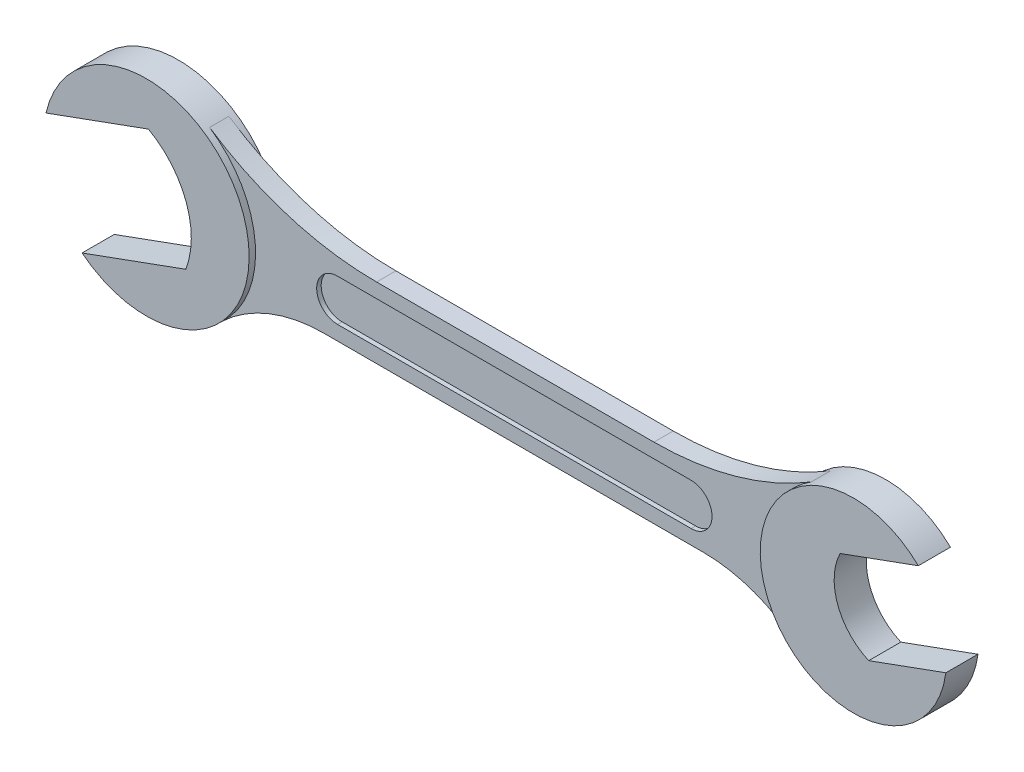
ISO-10303-21;
HEADER;
FILE_DESCRIPTION(('STEP AP214'),'2;1');
FILE_NAME('part.step','',(''),(''),'','','');
FILE_SCHEMA(('AUTOMOTIVE_DESIGN { 1 0 10303 214 1 1 1 1 }'));
ENDSEC;
DATA;
#1=APPLICATION_CONTEXT('core data for automotive mechanical design processes');
#2=APPLICATION_PROTOCOL_DEFINITION('international standard','automotive_design',2000,#1);
#3=PRODUCT_CONTEXT('',#1,'mechanical');
#4=PRODUCT('Part','Part','',(#3));
#5=PRODUCT_RELATED_PRODUCT_CATEGORY('part','',(#4));
#6=PRODUCT_DEFINITION_FORMATION('','',#4);
#7=PRODUCT_DEFINITION_CONTEXT('part definition',#1,'design');
#8=PRODUCT_DEFINITION('design','',#6,#7);
#9=PRODUCT_DEFINITION_SHAPE('','',#8);
#10=(LENGTH_UNIT() NAMED_UNIT(*) SI_UNIT(.MILLI.,.METRE.));
#11=(NAMED_UNIT(*) PLANE_ANGLE_UNIT() SI_UNIT($,.RADIAN.));
#12=(NAMED_UNIT(*) SI_UNIT($,.STERADIAN.) SOLID_ANGLE_UNIT());
#13=UNCERTAINTY_MEASURE_WITH_UNIT(LENGTH_MEASURE(1.E-05),#10,'distance_accuracy_value','');
#14=(GEOMETRIC_REPRESENTATION_CONTEXT(3) GLOBAL_UNCERTAINTY_ASSIGNED_CONTEXT((#13)) GLOBAL_UNIT_ASSIGNED_CONTEXT((#10,
#11,#12)) REPRESENTATION_CONTEXT('',''));
#15=CARTESIAN_POINT('',(0.,0.,0.));
#16=DIRECTION('',(0.,0.,1.));
#17=DIRECTION('',(1.,0.,0.));
#18=AXIS2_PLACEMENT_3D('',#15,#16,#17);
#19=CARTESIAN_POINT('',(0.,0.,3.));
#20=DIRECTION('',(0.,0.,1.));
#21=DIRECTION('',(1.,0.,0.));
#22=AXIS2_PLACEMENT_3D('',#19,#20,#21);
#23=PLANE('',#22);
#24=CARTESIAN_POINT('',(83.7536685908511,0.,3.));
#25=DIRECTION('',(0.,0.,1.));
#26=DIRECTION('',(1.,0.,0.));
#27=AXIS2_PLACEMENT_3D('',#24,#25,#26);
#28=CIRCLE('',#27,3.25);
#29=CARTESIAN_POINT('',(83.7536685908511,-3.25,3.));
#30=VERTEX_POINT('',#29);
#31=CARTESIAN_POINT('',(83.7536685908511,3.25,3.));
#32=VERTEX_POINT('',#31);
#33=EDGE_CURVE('E66',#30,#32,#28,.T.);
#34=ORIENTED_EDGE('',*,*,#33,.F.);
#35=DIRECTION('',(0.99999999999983,5.83857538673517E-07,0.));
#36=VECTOR('',#35,1.);
#37=CARTESIAN_POINT('',(83.7536685908511,-3.25,3.));
#38=LINE('',#37,#36);
#39=CARTESIAN_POINT('',(28.7536685908511,-3.25003211216463,3.));
#40=VERTEX_POINT('',#39);
#41=EDGE_CURVE('E241',#40,#30,#38,.T.);
#42=ORIENTED_EDGE('',*,*,#41,.F.);
#43=CARTESIAN_POINT('',(28.7536685908511,0.,3.));
#44=DIRECTION('',(0.,0.,1.));
#45=DIRECTION('',(1.,0.,0.));
#46=AXIS2_PLACEMENT_3D('',#43,#44,#45);
#47=CIRCLE('',#46,3.25003211216463);
#48=CARTESIAN_POINT('',(28.7681160854874,3.25,3.));
#49=VERTEX_POINT('',#48);
#50=EDGE_CURVE('E259',#49,#40,#47,.T.);
#51=ORIENTED_EDGE('',*,*,#50,.F.);
#52=DIRECTION('',(-1.,0.,0.));
#53=VECTOR('',#52,1.);
#54=CARTESIAN_POINT('',(28.7681160854874,3.25,3.));
#55=LINE('',#54,#53);
#56=EDGE_CURVE('E258',#32,#49,#55,.T.);
#57=ORIENTED_EDGE('',*,*,#56,.F.);
#58=EDGE_LOOP('',(#34,#42,#51,#57));
#59=FACE_BOUND('',#58,.T.);
#60=CARTESIAN_POINT('',(85.6278847860921,-28.5,3.));
#61=DIRECTION('',(0.,0.,1.));
#62=DIRECTION('',(1.,0.,0.));
#63=AXIS2_PLACEMENT_3D('',#60,#61,#62);
#64=CIRCLE('',#63,23.);
#65=CARTESIAN_POINT('',(100.576115450622,-11.02,3.));
#66=VERTEX_POINT('',#65);
#67=CARTESIAN_POINT('',(85.6278847860921,-5.5,3.));
#68=VERTEX_POINT('',#67);
#69=EDGE_CURVE('E341',#66,#68,#64,.T.);
#70=ORIENTED_EDGE('',*,*,#69,.F.);
#71=CARTESIAN_POINT('',(110.,0.,3.));
#72=DIRECTION('',(0.,0.,1.));
#73=DIRECTION('',(1.,0.,0.));
#74=AXIS2_PLACEMENT_3D('',#71,#72,#73);
#75=CIRCLE('',#74,14.5);
#76=CARTESIAN_POINT('',(102.447920260758,12.3780487804878,3.));
#77=VERTEX_POINT('',#76);
#78=EDGE_CURVE('E11',#66,#77,#75,.F.);
#79=ORIENTED_EDGE('',*,*,#78,.T.);
#80=CARTESIAN_POINT('',(77.9687652439061,52.5,3.));
#81=DIRECTION('',(0.,0.,1.));
#82=DIRECTION('',(1.,0.,0.));
#83=AXIS2_PLACEMENT_3D('',#80,#81,#82);
#84=CIRCLE('',#83,47.);
#85=CARTESIAN_POINT('',(77.9687652439086,5.5,3.));
#86=VERTEX_POINT('',#85);
#87=EDGE_CURVE('E327',#77,#86,#84,.F.);
#88=ORIENTED_EDGE('',*,*,#87,.T.);
#89=DIRECTION('',(1.,0.,0.));
#90=VECTOR('',#89,1.);
#91=CARTESIAN_POINT('',(0.,5.5,3.));
#92=LINE('',#91,#90);
#93=CARTESIAN_POINT('',(34.8245602987317,5.5,3.));
#94=VERTEX_POINT('',#93);
#95=EDGE_CURVE('E329',#94,#86,#92,.T.);
#96=ORIENTED_EDGE('',*,*,#95,.F.);
#97=CARTESIAN_POINT('',(34.8245602987317,52.5,3.));
#98=DIRECTION('',(0.,0.,1.));
#99=DIRECTION('',(1.,0.,0.));
#100=AXIS2_PLACEMENT_3D('',#97,#98,#99);
#101=CIRCLE('',#100,47.);
#102=CARTESIAN_POINT('',(8.84433277428107,13.3333333333333,3.));
#103=VERTEX_POINT('',#102);
#104=EDGE_CURVE('E331',#94,#103,#101,.F.);
#105=ORIENTED_EDGE('',*,*,#104,.T.);
#106=CARTESIAN_POINT('',(0.,0.,3.));
#107=DIRECTION('',(0.,0.,1.));
#108=DIRECTION('',(1.,0.,0.));
#109=AXIS2_PLACEMENT_3D('',#106,#107,#108);
#110=CIRCLE('',#109,16.);
#111=CARTESIAN_POINT('',(10.9219934457224,-11.6923076923077,3.));
#112=VERTEX_POINT('',#111);
#113=EDGE_CURVE('E315',#112,#103,#110,.T.);
#114=ORIENTED_EDGE('',*,*,#113,.F.);
#115=CARTESIAN_POINT('',(26.6223590239483,-28.5,3.));
#116=DIRECTION('',(0.,0.,1.));
#117=DIRECTION('',(1.,0.,0.));
#118=AXIS2_PLACEMENT_3D('',#115,#116,#117);
#119=CIRCLE('',#118,23.);
#120=CARTESIAN_POINT('',(26.6223590239447,-5.5,3.));
#121=VERTEX_POINT('',#120);
#122=EDGE_CURVE('E337',#121,#112,#119,.T.);
#123=ORIENTED_EDGE('',*,*,#122,.F.);
#124=DIRECTION('',(1.,0.,0.));
#125=VECTOR('',#124,1.);
#126=CARTESIAN_POINT('',(0.,-5.5,3.));
#127=LINE('',#126,#125);
#128=EDGE_CURVE('E339',#121,#68,#127,.T.);
#129=ORIENTED_EDGE('',*,*,#128,.T.);
#130=EDGE_LOOP('',(#70,#79,#88,#96,#105,#114,#123,#129));
#131=FACE_BOUND('',#130,.T.);
#132=ADVANCED_FACE('F43',(#59,#131),#23,.T.);
#133=CARTESIAN_POINT('',(0.,0.,0.));
#134=DIRECTION('',(0.,0.,1.));
#135=DIRECTION('',(1.,0.,0.));
#136=AXIS2_PLACEMENT_3D('',#133,#134,#135);
#137=PLANE('',#136);
#138=DIRECTION('',(-1.,0.,0.));
#139=VECTOR('',#138,1.);
#140=CARTESIAN_POINT('',(83.6251219050184,-3.24999999999999,0.));
#141=LINE('',#140,#139);
#142=CARTESIAN_POINT('',(83.6251219050184,-3.24999999999999,0.));
#143=VERTEX_POINT('',#142);
#144=CARTESIAN_POINT('',(28.6251219050184,-3.25,0.));
#145=VERTEX_POINT('',#144);
#146=EDGE_CURVE('E235',#143,#145,#141,.T.);
#147=ORIENTED_EDGE('',*,*,#146,.F.);
#148=CARTESIAN_POINT('',(83.6251219050184,0.,0.));
#149=DIRECTION('',(0.,0.,-1.));
#150=DIRECTION('',(-1.,0.,0.));
#151=AXIS2_PLACEMENT_3D('',#148,#149,#150);
#152=CIRCLE('',#151,3.24999999999999);
#153=CARTESIAN_POINT('',(83.6251219050184,3.24999999999999,0.));
#154=VERTEX_POINT('',#153);
#155=EDGE_CURVE('E59',#154,#143,#152,.T.);
#156=ORIENTED_EDGE('',*,*,#155,.F.);
#157=DIRECTION('',(1.,0.,0.));
#158=VECTOR('',#157,1.);
#159=CARTESIAN_POINT('',(83.6251219050184,3.24999999999999,0.));
#160=LINE('',#159,#158);
#161=CARTESIAN_POINT('',(28.6251219050184,3.25,0.));
#162=VERTEX_POINT('',#161);
#163=EDGE_CURVE('E224',#162,#154,#160,.T.);
#164=ORIENTED_EDGE('',*,*,#163,.F.);
#165=CARTESIAN_POINT('',(28.6251219050184,0.,0.));
#166=DIRECTION('',(0.,0.,-1.));
#167=DIRECTION('',(-1.,0.,0.));
#168=AXIS2_PLACEMENT_3D('',#165,#166,#167);
#169=CIRCLE('',#168,3.25);
#170=EDGE_CURVE('E227',#145,#162,#169,.T.);
#171=ORIENTED_EDGE('',*,*,#170,.F.);
#172=EDGE_LOOP('',(#147,#156,#164,#171));
#173=FACE_BOUND('',#172,.T.);
#174=CARTESIAN_POINT('',(110.,0.,0.));
#175=DIRECTION('',(0.,0.,-1.));
#176=DIRECTION('',(-1.,0.,0.));
#177=AXIS2_PLACEMENT_3D('',#174,#175,#176);
#178=CIRCLE('',#177,14.5);
#179=CARTESIAN_POINT('',(100.576115450622,-11.02,0.));
#180=VERTEX_POINT('',#179);
#181=CARTESIAN_POINT('',(102.447920260758,12.3780487804878,0.));
#182=VERTEX_POINT('',#181);
#183=EDGE_CURVE('E283',#180,#182,#178,.T.);
#184=ORIENTED_EDGE('',*,*,#183,.F.);
#185=CARTESIAN_POINT('',(85.6278847860921,-28.5,0.));
#186=DIRECTION('',(0.,0.,1.));
#187=DIRECTION('',(1.,0.,0.));
#188=AXIS2_PLACEMENT_3D('',#185,#186,#187);
#189=CIRCLE('',#188,23.);
#190=CARTESIAN_POINT('',(85.6278847860921,-5.5,0.));
#191=VERTEX_POINT('',#190);
#192=EDGE_CURVE('E332',#180,#191,#189,.T.);
#193=ORIENTED_EDGE('',*,*,#192,.T.);
#194=DIRECTION('',(1.,0.,0.));
#195=VECTOR('',#194,1.);
#196=CARTESIAN_POINT('',(0.,-5.5,0.));
#197=LINE('',#196,#195);
#198=CARTESIAN_POINT('',(26.6223590239447,-5.5,0.));
#199=VERTEX_POINT('',#198);
#200=EDGE_CURVE('E356',#199,#191,#197,.T.);
#201=ORIENTED_EDGE('',*,*,#200,.F.);
#202=CARTESIAN_POINT('',(26.6223590239483,-28.5,0.));
#203=DIRECTION('',(0.,0.,1.));
#204=DIRECTION('',(1.,0.,0.));
#205=AXIS2_PLACEMENT_3D('',#202,#203,#204);
#206=CIRCLE('',#205,23.);
#207=CARTESIAN_POINT('',(10.9219934457224,-11.6923076923077,0.));
#208=VERTEX_POINT('',#207);
#209=EDGE_CURVE('E353',#199,#208,#206,.T.);
#210=ORIENTED_EDGE('',*,*,#209,.T.);
#211=CARTESIAN_POINT('',(0.,0.,0.));
#212=DIRECTION('',(0.,0.,-1.));
#213=DIRECTION('',(-1.,0.,0.));
#214=AXIS2_PLACEMENT_3D('',#211,#212,#213);
#215=CIRCLE('',#214,16.);
#216=CARTESIAN_POINT('',(8.84433277428106,13.3333333333333,0.));
#217=VERTEX_POINT('',#216);
#218=EDGE_CURVE('E51',#217,#208,#215,.T.);
#219=ORIENTED_EDGE('',*,*,#218,.F.);
#220=CARTESIAN_POINT('',(34.8245602987317,52.5,0.));
#221=DIRECTION('',(0.,0.,1.));
#222=DIRECTION('',(1.,0.,0.));
#223=AXIS2_PLACEMENT_3D('',#220,#221,#222);
#224=CIRCLE('',#223,47.);
#225=CARTESIAN_POINT('',(34.8245602987317,5.5,0.));
#226=VERTEX_POINT('',#225);
#227=EDGE_CURVE('E348',#226,#217,#224,.F.);
#228=ORIENTED_EDGE('',*,*,#227,.F.);
#229=DIRECTION('',(1.,0.,0.));
#230=VECTOR('',#229,1.);
#231=CARTESIAN_POINT('',(0.,5.5,0.));
#232=LINE('',#231,#230);
#233=CARTESIAN_POINT('',(77.9687652439086,5.5,0.));
#234=VERTEX_POINT('',#233);
#235=EDGE_CURVE('E350',#226,#234,#232,.T.);
#236=ORIENTED_EDGE('',*,*,#235,.T.);
#237=CARTESIAN_POINT('',(77.9687652439061,52.5,0.));
#238=DIRECTION('',(0.,0.,1.));
#239=DIRECTION('',(1.,0.,0.));
#240=AXIS2_PLACEMENT_3D('',#237,#238,#239);
#241=CIRCLE('',#240,47.);
#242=EDGE_CURVE('E322',#182,#234,#241,.F.);
#243=ORIENTED_EDGE('',*,*,#242,.F.);
#244=EDGE_LOOP('',(#184,#193,#201,#210,#219,#228,#236,#243));
#245=FACE_BOUND('',#244,.T.);
#246=ADVANCED_FACE('F422',(#173,#245),#137,.F.);
#247=CARTESIAN_POINT('',(10.7035037567005,-29.4076348820317,3.));
#248=DIRECTION('',(0.342020143310785,-0.939692620791326,0.));
#249=DIRECTION('',(0.939692620791326,0.342020143310785,0.));
#250=AXIS2_PLACEMENT_3D('',#247,#248,#249);
#251=PLANE('',#250);
#252=DIRECTION('',(0.,0.,-1.));
#253=VECTOR('',#252,1.);
#254=CARTESIAN_POINT('',(107.927329676916,5.97894381266167,3.));
#255=LINE('',#254,#253);
#256=CARTESIAN_POINT('',(107.927329676916,5.97894381266167,4.));
#257=VERTEX_POINT('',#256);
#258=CARTESIAN_POINT('',(107.927329676916,5.97894381266167,-1.));
#259=VERTEX_POINT('',#258);
#260=EDGE_CURVE('E343',#257,#259,#255,.T.);
#261=ORIENTED_EDGE('',*,*,#260,.T.);
#262=DIRECTION('',(-0.939692620791326,-0.342020143310785,0.));
#263=VECTOR('',#262,1.);
#264=CARTESIAN_POINT('',(107.927329676916,5.97894381266167,-1.));
#265=LINE('',#264,#263);
#266=CARTESIAN_POINT('',(120.095812240616,10.4079092618175,-1.));
#267=VERTEX_POINT('',#266);
#268=EDGE_CURVE('E291',#267,#259,#265,.T.);
#269=ORIENTED_EDGE('',*,*,#268,.F.);
#270=DIRECTION('',(0.,0.,-1.));
#271=VECTOR('',#270,1.);
#272=CARTESIAN_POINT('',(120.095812240616,10.4079092618175,3.));
#273=LINE('',#272,#271);
#274=CARTESIAN_POINT('',(120.095812240616,10.4079092618175,4.));
#275=VERTEX_POINT('',#274);
#276=EDGE_CURVE('E330',#275,#267,#273,.T.);
#277=ORIENTED_EDGE('',*,*,#276,.F.);
#278=DIRECTION('',(0.939692620791326,0.342020143310785,0.));
#279=VECTOR('',#278,1.);
#280=CARTESIAN_POINT('',(107.927329676916,5.97894381266167,4.));
#281=LINE('',#280,#279);
#282=EDGE_CURVE('E273',#257,#275,#281,.T.);
#283=ORIENTED_EDGE('',*,*,#282,.F.);
#284=EDGE_LOOP('',(#261,#269,#277,#283));
#285=FACE_BOUND('',#284,.T.);
#286=ADVANCED_FACE('F44',(#285),#251,.T.);
#287=CARTESIAN_POINT('',(77.9687652439061,52.5,3.));
#288=DIRECTION('',(0.,0.,-1.));
#289=DIRECTION('',(-1.,0.,0.));
#290=AXIS2_PLACEMENT_3D('',#287,#288,#289);
#291=CYLINDRICAL_SURFACE('',#290,47.);
#292=ORIENTED_EDGE('',*,*,#242,.T.);
#293=DIRECTION('',(0.,0.,-1.));
#294=VECTOR('',#293,1.);
#295=CARTESIAN_POINT('',(77.9687652439086,5.5,3.));
#296=LINE('',#295,#294);
#297=EDGE_CURVE('E386',#86,#234,#296,.T.);
#298=ORIENTED_EDGE('',*,*,#297,.F.);
#299=ORIENTED_EDGE('',*,*,#87,.F.);
#300=DIRECTION('',(0.,0.,-1.));
#301=VECTOR('',#300,1.);
#302=CARTESIAN_POINT('',(102.447920260758,12.3780487804878,3.));
#303=LINE('',#302,#301);
#304=EDGE_CURVE('E392',#77,#182,#303,.T.);
#305=ORIENTED_EDGE('',*,*,#304,.T.);
#306=EDGE_LOOP('',(#292,#298,#299,#305));
#307=FACE_BOUND('',#306,.T.);
#308=ADVANCED_FACE('F480',(#307),#291,.F.);
#309=CARTESIAN_POINT('',(0.,5.5,3.));
#310=DIRECTION('',(0.,1.,0.));
#311=DIRECTION('',(0.,0.,1.));
#312=AXIS2_PLACEMENT_3D('',#309,#310,#311);
#313=PLANE('',#312);
#314=ORIENTED_EDGE('',*,*,#235,.F.);
#315=DIRECTION('',(0.,0.,-1.));
#316=VECTOR('',#315,1.);
#317=CARTESIAN_POINT('',(34.8245602987317,5.5,3.));
#318=LINE('',#317,#316);
#319=EDGE_CURVE('E390',#94,#226,#318,.T.);
#320=ORIENTED_EDGE('',*,*,#319,.F.);
#321=ORIENTED_EDGE('',*,*,#95,.T.);
#322=ORIENTED_EDGE('',*,*,#297,.T.);
#323=EDGE_LOOP('',(#314,#320,#321,#322));
#324=FACE_BOUND('',#323,.T.);
#325=ADVANCED_FACE('F475',(#324),#313,.T.);
#326=CARTESIAN_POINT('',(34.8245602987317,52.5,3.));
#327=DIRECTION('',(0.,0.,-1.));
#328=DIRECTION('',(-1.,0.,0.));
#329=AXIS2_PLACEMENT_3D('',#326,#327,#328);
#330=CYLINDRICAL_SURFACE('',#329,47.);
#331=ORIENTED_EDGE('',*,*,#227,.T.);
#332=DIRECTION('',(0.,0.,-1.));
#333=VECTOR('',#332,1.);
#334=CARTESIAN_POINT('',(8.84433277428107,13.3333333333333,3.));
#335=LINE('',#334,#333);
#336=EDGE_CURVE('E383',#103,#217,#335,.T.);
#337=ORIENTED_EDGE('',*,*,#336,.F.);
#338=ORIENTED_EDGE('',*,*,#104,.F.);
#339=ORIENTED_EDGE('',*,*,#319,.T.);
#340=EDGE_LOOP('',(#331,#337,#338,#339));
#341=FACE_BOUND('',#340,.T.);
#342=ADVANCED_FACE('F469',(#341),#330,.F.);
#343=CARTESIAN_POINT('',(-2.96625027922472,8.14970566262087,3.));
#344=DIRECTION('',(-0.34202014332567,0.939692620785908,0.));
#345=DIRECTION('',(-0.939692620785908,-0.34202014332567,0.));
#346=AXIS2_PLACEMENT_3D('',#343,#344,#345);
#347=PLANE('',#346);
#348=DIRECTION('',(0.,0.,-1.));
#349=VECTOR('',#348,1.);
#350=CARTESIAN_POINT('',(-15.6009638229452,3.55104601422654,3.));
#351=LINE('',#350,#349);
#352=CARTESIAN_POINT('',(-15.6009638229452,3.55104601422654,4.));
#353=VERTEX_POINT('',#352);
#354=CARTESIAN_POINT('',(-15.6009638229452,3.55104601422654,-1.));
#355=VERTEX_POINT('',#354);
#356=EDGE_CURVE('E385',#353,#355,#351,.T.);
#357=ORIENTED_EDGE('',*,*,#356,.T.);
#358=DIRECTION('',(-0.939692620785908,-0.34202014332567,0.));
#359=VECTOR('',#358,1.);
#360=CARTESIAN_POINT('',(0.335793670547545,9.35155137257678,-1.));
#361=LINE('',#360,#359);
#362=CARTESIAN_POINT('',(0.335793670547545,9.35155137257678,-1.));
#363=VERTEX_POINT('',#362);
#364=EDGE_CURVE('E301',#363,#355,#361,.T.);
#365=ORIENTED_EDGE('',*,*,#364,.F.);
#366=DIRECTION('',(0.,0.,-1.));
#367=VECTOR('',#366,1.);
#368=CARTESIAN_POINT('',(0.335793670547545,9.35155137257678,3.));
#369=LINE('',#368,#367);
#370=CARTESIAN_POINT('',(0.335793670547545,9.35155137257678,4.));
#371=VERTEX_POINT('',#370);
#372=EDGE_CURVE('E379',#371,#363,#369,.T.);
#373=ORIENTED_EDGE('',*,*,#372,.F.);
#374=DIRECTION('',(0.939692620785908,0.34202014332567,0.));
#375=VECTOR('',#374,1.);
#376=CARTESIAN_POINT('',(-15.6009638229452,3.55104601422654,4.));
#377=LINE('',#376,#375);
#378=EDGE_CURVE('E312',#353,#371,#377,.T.);
#379=ORIENTED_EDGE('',*,*,#378,.F.);
#380=EDGE_LOOP('',(#357,#365,#373,#379));
#381=FACE_BOUND('',#380,.T.);
#382=ADVANCED_FACE('F466',(#381),#347,.F.);
#383=CARTESIAN_POINT('',(-6.,-2.,3.));
#384=DIRECTION('',(0.,0.,-1.));
#385=DIRECTION('',(-1.,0.,0.));
#386=AXIS2_PLACEMENT_3D('',#383,#384,#385);
#387=CYLINDRICAL_SURFACE('',#386,13.);
#388=ORIENTED_EDGE('',*,*,#372,.T.);
#389=CARTESIAN_POINT('',(-6.,-2.,-1.));
#390=DIRECTION('',(0.,0.,1.));
#391=DIRECTION('',(1.,0.,0.));
#392=AXIS2_PLACEMENT_3D('',#389,#390,#391);
#393=CIRCLE('',#392,13.);
#394=CARTESIAN_POINT('',(6.15013610708393,-6.62322318078366,-1.));
#395=VERTEX_POINT('',#394);
#396=EDGE_CURVE('E297',#395,#363,#393,.T.);
#397=ORIENTED_EDGE('',*,*,#396,.F.);
#398=DIRECTION('',(0.,0.,-1.));
#399=VECTOR('',#398,1.);
#400=CARTESIAN_POINT('',(6.15013610708393,-6.62322318078366,3.));
#401=LINE('',#400,#399);
#402=CARTESIAN_POINT('',(6.15013610708393,-6.62322318078366,4.));
#403=VERTEX_POINT('',#402);
#404=EDGE_CURVE('E378',#403,#395,#401,.T.);
#405=ORIENTED_EDGE('',*,*,#404,.F.);
#406=CARTESIAN_POINT('',(-6.00000000000002,-2.,4.));
#407=DIRECTION('',(0.,0.,-1.));
#408=DIRECTION('',(-1.,0.,0.));
#409=AXIS2_PLACEMENT_3D('',#406,#407,#408);
#410=CIRCLE('',#409,13.);
#411=EDGE_CURVE('E318',#371,#403,#410,.T.);
#412=ORIENTED_EDGE('',*,*,#411,.F.);
#413=EDGE_LOOP('',(#388,#397,#405,#412));
#414=FACE_BOUND('',#413,.T.);
#415=ADVANCED_FACE('F465',(#414),#387,.F.);
#416=CARTESIAN_POINT('',(2.84809215731166,-7.82506889073957,3.));
#417=DIRECTION('',(0.342020143325669,-0.939692620785908,0.));
#418=DIRECTION('',(0.939692620785908,0.342020143325669,0.));
#419=AXIS2_PLACEMENT_3D('',#416,#417,#418);
#420=PLANE('',#419);
#421=ORIENTED_EDGE('',*,*,#404,.T.);
#422=DIRECTION('',(0.939692620785908,0.342020143325669,0.));
#423=VECTOR('',#422,1.);
#424=CARTESIAN_POINT('',(6.15013610708393,-6.62322318078366,-1.));
#425=LINE('',#424,#423);
#426=CARTESIAN_POINT('',(-9.99020934928993,-12.4978284976775,-1.));
#427=VERTEX_POINT('',#426);
#428=EDGE_CURVE('E307',#427,#395,#425,.T.);
#429=ORIENTED_EDGE('',*,*,#428,.F.);
#430=DIRECTION('',(0.,0.,-1.));
#431=VECTOR('',#430,1.);
#432=CARTESIAN_POINT('',(-9.99020934928993,-12.4978284976775,3.));
#433=LINE('',#432,#431);
#434=CARTESIAN_POINT('',(-9.99020934928993,-12.4978284976775,4.));
#435=VERTEX_POINT('',#434);
#436=EDGE_CURVE('E376',#435,#427,#433,.T.);
#437=ORIENTED_EDGE('',*,*,#436,.F.);
#438=DIRECTION('',(-0.939692620785908,-0.342020143325669,0.));
#439=VECTOR('',#438,1.);
#440=CARTESIAN_POINT('',(-9.99020934928993,-12.4978284976775,4.));
#441=LINE('',#440,#439);
#442=EDGE_CURVE('E321',#403,#435,#441,.T.);
#443=ORIENTED_EDGE('',*,*,#442,.F.);
#444=EDGE_LOOP('',(#421,#429,#437,#443));
#445=FACE_BOUND('',#444,.T.);
#446=ADVANCED_FACE('F456',(#445),#420,.F.);
#447=CARTESIAN_POINT('',(0.,0.,3.));
#448=DIRECTION('',(0.,0.,-1.));
#449=DIRECTION('',(-1.,0.,0.));
#450=AXIS2_PLACEMENT_3D('',#447,#448,#449);
#451=CYLINDRICAL_SURFACE('',#450,16.);
#452=CARTESIAN_POINT('',(0.,0.,-1.));
#453=DIRECTION('',(0.,0.,-1.));
#454=DIRECTION('',(-1.,0.,0.));
#455=AXIS2_PLACEMENT_3D('',#452,#453,#454);
#456=CIRCLE('',#455,16.);
#457=EDGE_CURVE('E303',#355,#427,#456,.T.);
#458=ORIENTED_EDGE('',*,*,#457,.F.);
#459=ORIENTED_EDGE('',*,*,#356,.F.);
#460=CARTESIAN_POINT('',(0.,0.,4.));
#461=DIRECTION('',(0.,0.,1.));
#462=DIRECTION('',(1.,0.,0.));
#463=AXIS2_PLACEMENT_3D('',#460,#461,#462);
#464=CIRCLE('',#463,16.);
#465=EDGE_CURVE('E309',#435,#353,#464,.T.);
#466=ORIENTED_EDGE('',*,*,#465,.F.);
#467=ORIENTED_EDGE('',*,*,#436,.T.);
#468=EDGE_LOOP('',(#458,#459,#466,#467));
#469=FACE_BOUND('',#468,.T.);
#470=ORIENTED_EDGE('',*,*,#336,.T.);
#471=ORIENTED_EDGE('',*,*,#218,.T.);
#472=DIRECTION('',(0.,0.,-1.));
#473=VECTOR('',#472,1.);
#474=CARTESIAN_POINT('',(10.9219934457224,-11.6923076923077,3.));
#475=LINE('',#474,#473);
#476=EDGE_CURVE('E373',#112,#208,#475,.T.);
#477=ORIENTED_EDGE('',*,*,#476,.F.);
#478=ORIENTED_EDGE('',*,*,#113,.T.);
#479=EDGE_LOOP('',(#470,#471,#477,#478));
#480=FACE_BOUND('',#479,.T.);
#481=ADVANCED_FACE('F453',(#469,#480),#451,.T.);
#482=CARTESIAN_POINT('',(26.6223590239483,-28.5,3.));
#483=DIRECTION('',(0.,0.,-1.));
#484=DIRECTION('',(-1.,0.,0.));
#485=AXIS2_PLACEMENT_3D('',#482,#483,#484);
#486=CYLINDRICAL_SURFACE('',#485,23.);
#487=ORIENTED_EDGE('',*,*,#209,.F.);
#488=DIRECTION('',(0.,0.,-1.));
#489=VECTOR('',#488,1.);
#490=CARTESIAN_POINT('',(26.6223590239447,-5.5,3.));
#491=LINE('',#490,#489);
#492=EDGE_CURVE('E371',#121,#199,#491,.T.);
#493=ORIENTED_EDGE('',*,*,#492,.F.);
#494=ORIENTED_EDGE('',*,*,#122,.T.);
#495=ORIENTED_EDGE('',*,*,#476,.T.);
#496=EDGE_LOOP('',(#487,#493,#494,#495));
#497=FACE_BOUND('',#496,.T.);
#498=ADVANCED_FACE('F446',(#497),#486,.F.);
#499=CARTESIAN_POINT('',(0.,-5.5,3.));
#500=DIRECTION('',(0.,1.,0.));
#501=DIRECTION('',(-1.,0.,0.));
#502=AXIS2_PLACEMENT_3D('',#499,#500,#501);
#503=PLANE('',#502);
#504=ORIENTED_EDGE('',*,*,#200,.T.);
#505=DIRECTION('',(0.,0.,-1.));
#506=VECTOR('',#505,1.);
#507=CARTESIAN_POINT('',(85.6278847860921,-5.5,3.));
#508=LINE('',#507,#506);
#509=EDGE_CURVE('E369',#68,#191,#508,.T.);
#510=ORIENTED_EDGE('',*,*,#509,.F.);
#511=ORIENTED_EDGE('',*,*,#128,.F.);
#512=ORIENTED_EDGE('',*,*,#492,.T.);
#513=EDGE_LOOP('',(#504,#510,#511,#512));
#514=FACE_BOUND('',#513,.T.);
#515=ADVANCED_FACE('F447',(#514),#503,.F.);
#516=CARTESIAN_POINT('',(85.6278847860921,-28.5,3.));
#517=DIRECTION('',(0.,0.,-1.));
#518=DIRECTION('',(-1.,0.,0.));
#519=AXIS2_PLACEMENT_3D('',#516,#517,#518);
#520=CYLINDRICAL_SURFACE('',#519,23.);
#521=ORIENTED_EDGE('',*,*,#192,.F.);
#522=DIRECTION('',(0.,0.,-1.));
#523=VECTOR('',#522,1.);
#524=CARTESIAN_POINT('',(100.576115450622,-11.02,3.));
#525=LINE('',#524,#523);
#526=EDGE_CURVE('E368',#66,#180,#525,.T.);
#527=ORIENTED_EDGE('',*,*,#526,.F.);
#528=ORIENTED_EDGE('',*,*,#69,.T.);
#529=ORIENTED_EDGE('',*,*,#509,.T.);
#530=EDGE_LOOP('',(#521,#527,#528,#529));
#531=FACE_BOUND('',#530,.T.);
#532=ADVANCED_FACE('F444',(#531),#520,.F.);
#533=CARTESIAN_POINT('',(110.,0.,3.));
#534=DIRECTION('',(0.,0.,-1.));
#535=DIRECTION('',(-1.,0.,0.));
#536=AXIS2_PLACEMENT_3D('',#533,#534,#535);
#537=CYLINDRICAL_SURFACE('',#536,14.5);
#538=DIRECTION('',(0.,0.,-1.));
#539=VECTOR('',#538,1.);
#540=CARTESIAN_POINT('',(124.379255247521,-1.86735602567682,3.));
#541=LINE('',#540,#539);
#542=CARTESIAN_POINT('',(124.379255247521,-1.86735602567682,4.));
#543=VERTEX_POINT('',#542);
#544=CARTESIAN_POINT('',(124.379255247521,-1.86735602567682,-1.));
#545=VERTEX_POINT('',#544);
#546=EDGE_CURVE('E365',#543,#545,#541,.T.);
#547=ORIENTED_EDGE('',*,*,#546,.F.);
#548=CARTESIAN_POINT('',(110.,0.,4.));
#549=DIRECTION('',(0.,0.,1.));
#550=DIRECTION('',(1.,0.,0.));
#551=AXIS2_PLACEMENT_3D('',#548,#549,#550);
#552=CIRCLE('',#551,14.5);
#553=EDGE_CURVE('E280',#275,#543,#552,.T.);
#554=ORIENTED_EDGE('',*,*,#553,.F.);
#555=ORIENTED_EDGE('',*,*,#276,.T.);
#556=CARTESIAN_POINT('',(110.,0.,-1.));
#557=DIRECTION('',(0.,0.,-1.));
#558=DIRECTION('',(-1.,0.,0.));
#559=AXIS2_PLACEMENT_3D('',#556,#557,#558);
#560=CIRCLE('',#559,14.5);
#561=EDGE_CURVE('E289',#545,#267,#560,.T.);
#562=ORIENTED_EDGE('',*,*,#561,.F.);
#563=EDGE_LOOP('',(#547,#554,#555,#562));
#564=FACE_BOUND('',#563,.T.);
#565=ORIENTED_EDGE('',*,*,#526,.T.);
#566=ORIENTED_EDGE('',*,*,#183,.T.);
#567=ORIENTED_EDGE('',*,*,#304,.F.);
#568=ORIENTED_EDGE('',*,*,#78,.F.);
#569=EDGE_LOOP('',(#565,#566,#567,#568));
#570=FACE_BOUND('',#569,.T.);
#571=ADVANCED_FACE('F391',(#564,#570),#537,.T.);
#572=CARTESIAN_POINT('',(15.1497656197431,-41.6236389523214,3.));
#573=DIRECTION('',(-0.342020143310813,0.939692620791315,0.));
#574=DIRECTION('',(-0.939692620791316,-0.342020143310813,0.));
#575=AXIS2_PLACEMENT_3D('',#572,#573,#574);
#576=PLANE('',#575);
#577=ORIENTED_EDGE('',*,*,#546,.T.);
#578=DIRECTION('',(0.939692620791316,0.342020143310813,0.));
#579=VECTOR('',#578,1.);
#580=CARTESIAN_POINT('',(112.373591540149,-6.23706025755531,-1.));
#581=LINE('',#580,#579);
#582=CARTESIAN_POINT('',(112.373591540149,-6.23706025755531,-1.));
#583=VERTEX_POINT('',#582);
#584=EDGE_CURVE('E290',#583,#545,#581,.T.);
#585=ORIENTED_EDGE('',*,*,#584,.F.);
#586=DIRECTION('',(0.,0.,-1.));
#587=VECTOR('',#586,1.);
#588=CARTESIAN_POINT('',(112.373591540149,-6.23706025755531,3.));
#589=LINE('',#588,#587);
#590=CARTESIAN_POINT('',(112.373591540149,-6.23706025755531,4.));
#591=VERTEX_POINT('',#590);
#592=EDGE_CURVE('E362',#591,#583,#589,.T.);
#593=ORIENTED_EDGE('',*,*,#592,.F.);
#594=DIRECTION('',(-0.939692620791316,-0.342020143310813,0.));
#595=VECTOR('',#594,1.);
#596=CARTESIAN_POINT('',(112.373591540149,-6.23706025755531,4.));
#597=LINE('',#596,#595);
#598=EDGE_CURVE('E278',#543,#591,#597,.T.);
#599=ORIENTED_EDGE('',*,*,#598,.F.);
#600=EDGE_LOOP('',(#577,#585,#593,#599));
#601=FACE_BOUND('',#600,.T.);
#602=ADVANCED_FACE('F409',(#601),#576,.T.);
#603=CARTESIAN_POINT('',(115.99999999941,2.0000000000001,3.));
#604=DIRECTION('',(0.,0.,-1.));
#605=DIRECTION('',(-1.,0.,0.));
#606=AXIS2_PLACEMENT_3D('',#603,#604,#605);
#607=CYLINDRICAL_SURFACE('',#606,9.);
#608=ORIENTED_EDGE('',*,*,#592,.T.);
#609=CARTESIAN_POINT('',(115.99999999941,2.00000000000009,-1.));
#610=DIRECTION('',(0.,0.,1.));
#611=DIRECTION('',(1.,0.,0.));
#612=AXIS2_PLACEMENT_3D('',#609,#610,#611);
#613=CIRCLE('',#612,9.00000000000001);
#614=EDGE_CURVE('E284',#259,#583,#613,.T.);
#615=ORIENTED_EDGE('',*,*,#614,.F.);
#616=ORIENTED_EDGE('',*,*,#260,.F.);
#617=CARTESIAN_POINT('',(115.99999999941,2.00000000000009,4.));
#618=DIRECTION('',(0.,0.,-1.));
#619=DIRECTION('',(1.,0.,0.));
#620=AXIS2_PLACEMENT_3D('',#617,#618,#619);
#621=CIRCLE('',#620,9.00000000000001);
#622=EDGE_CURVE('E266',#591,#257,#621,.T.);
#623=ORIENTED_EDGE('',*,*,#622,.F.);
#624=EDGE_LOOP('',(#608,#615,#616,#623));
#625=FACE_BOUND('',#624,.T.);
#626=ADVANCED_FACE('F407',(#625),#607,.F.);
#627=CARTESIAN_POINT('',(0.,0.,4.));
#628=DIRECTION('',(0.,0.,1.));
#629=DIRECTION('',(1.,0.,0.));
#630=AXIS2_PLACEMENT_3D('',#627,#628,#629);
#631=PLANE('',#630);
#632=ORIENTED_EDGE('',*,*,#465,.T.);
#633=ORIENTED_EDGE('',*,*,#378,.T.);
#634=ORIENTED_EDGE('',*,*,#411,.T.);
#635=ORIENTED_EDGE('',*,*,#442,.T.);
#636=EDGE_LOOP('',(#632,#633,#634,#635));
#637=FACE_BOUND('',#636,.T.);
#638=ADVANCED_FACE('F434',(#637),#631,.T.);
#639=CARTESIAN_POINT('',(-6.,-2.,-1.));
#640=DIRECTION('',(0.,0.,1.));
#641=DIRECTION('',(1.,0.,0.));
#642=AXIS2_PLACEMENT_3D('',#639,#640,#641);
#643=PLANE('',#642);
#644=ORIENTED_EDGE('',*,*,#396,.T.);
#645=ORIENTED_EDGE('',*,*,#364,.T.);
#646=ORIENTED_EDGE('',*,*,#457,.T.);
#647=ORIENTED_EDGE('',*,*,#428,.T.);
#648=EDGE_LOOP('',(#644,#645,#646,#647));
#649=FACE_BOUND('',#648,.T.);
#650=ADVANCED_FACE('F421',(#649),#643,.F.);
#651=CARTESIAN_POINT('',(115.99999999941,2.00000000000009,-1.));
#652=DIRECTION('',(0.,0.,1.));
#653=DIRECTION('',(1.,0.,0.));
#654=AXIS2_PLACEMENT_3D('',#651,#652,#653);
#655=PLANE('',#654);
#656=ORIENTED_EDGE('',*,*,#614,.T.);
#657=ORIENTED_EDGE('',*,*,#584,.T.);
#658=ORIENTED_EDGE('',*,*,#561,.T.);
#659=ORIENTED_EDGE('',*,*,#268,.T.);
#660=EDGE_LOOP('',(#656,#657,#658,#659));
#661=FACE_BOUND('',#660,.T.);
#662=ADVANCED_FACE('F402',(#661),#655,.F.);
#663=CARTESIAN_POINT('',(115.99999999941,2.00000000000009,4.));
#664=DIRECTION('',(0.,0.,1.));
#665=DIRECTION('',(1.,0.,0.));
#666=AXIS2_PLACEMENT_3D('',#663,#664,#665);
#667=PLANE('',#666);
#668=ORIENTED_EDGE('',*,*,#622,.T.);
#669=ORIENTED_EDGE('',*,*,#282,.T.);
#670=ORIENTED_EDGE('',*,*,#553,.T.);
#671=ORIENTED_EDGE('',*,*,#598,.T.);
#672=EDGE_LOOP('',(#668,#669,#670,#671));
#673=FACE_BOUND('',#672,.T.);
#674=ADVANCED_FACE('F411',(#673),#667,.T.);
#675=CARTESIAN_POINT('',(83.7536685908511,0.,2.3));
#676=DIRECTION('',(0.,0.,1.));
#677=DIRECTION('',(1.,0.,0.));
#678=AXIS2_PLACEMENT_3D('',#675,#676,#677);
#679=CYLINDRICAL_SURFACE('',#678,3.25);
#680=ORIENTED_EDGE('',*,*,#33,.T.);
#681=DIRECTION('',(0.,0.,1.));
#682=VECTOR('',#681,1.);
#683=CARTESIAN_POINT('',(83.7536685908511,3.25,2.3));
#684=LINE('',#683,#682);
#685=CARTESIAN_POINT('',(83.7536685908511,3.25,2.3));
#686=VERTEX_POINT('',#685);
#687=EDGE_CURVE('E255',#686,#32,#684,.T.);
#688=ORIENTED_EDGE('',*,*,#687,.F.);
#689=CARTESIAN_POINT('',(83.7536685908511,0.,2.3));
#690=DIRECTION('',(0.,0.,1.));
#691=DIRECTION('',(1.,0.,0.));
#692=AXIS2_PLACEMENT_3D('',#689,#690,#691);
#693=CIRCLE('',#692,3.25);
#694=CARTESIAN_POINT('',(83.7536685908511,-3.25,2.3));
#695=VERTEX_POINT('',#694);
#696=EDGE_CURVE('E242',#695,#686,#693,.T.);
#697=ORIENTED_EDGE('',*,*,#696,.F.);
#698=DIRECTION('',(0.,0.,1.));
#699=VECTOR('',#698,1.);
#700=CARTESIAN_POINT('',(83.7536685908511,-3.25,2.3));
#701=LINE('',#700,#699);
#702=EDGE_CURVE('E262',#695,#30,#701,.T.);
#703=ORIENTED_EDGE('',*,*,#702,.T.);
#704=EDGE_LOOP('',(#680,#688,#697,#703));
#705=FACE_BOUND('',#704,.T.);
#706=ADVANCED_FACE('F412',(#705),#679,.F.);
#707=CARTESIAN_POINT('',(83.7536685908511,-3.25,2.3));
#708=DIRECTION('',(5.83857538673517E-07,-0.999999999999829,0.));
#709=DIRECTION('',(0.99999999999983,5.83857538673517E-07,0.));
#710=AXIS2_PLACEMENT_3D('',#707,#708,#709);
#711=PLANE('',#710);
#712=ORIENTED_EDGE('',*,*,#41,.T.);
#713=ORIENTED_EDGE('',*,*,#702,.F.);
#714=DIRECTION('',(0.99999999999983,5.83857538673517E-07,0.));
#715=VECTOR('',#714,1.);
#716=CARTESIAN_POINT('',(83.7536685908511,-3.25,2.3));
#717=LINE('',#716,#715);
#718=CARTESIAN_POINT('',(28.7536685908511,-3.25003211216463,2.3));
#719=VERTEX_POINT('',#718);
#720=EDGE_CURVE('E253',#719,#695,#717,.T.);
#721=ORIENTED_EDGE('',*,*,#720,.F.);
#722=DIRECTION('',(0.,0.,1.));
#723=VECTOR('',#722,1.);
#724=CARTESIAN_POINT('',(28.7536685908511,-3.25003211216463,2.3));
#725=LINE('',#724,#723);
#726=EDGE_CURVE('E270',#719,#40,#725,.T.);
#727=ORIENTED_EDGE('',*,*,#726,.T.);
#728=EDGE_LOOP('',(#712,#713,#721,#727));
#729=FACE_BOUND('',#728,.T.);
#730=ADVANCED_FACE('F419',(#729),#711,.F.);
#731=CARTESIAN_POINT('',(28.7536685908511,0.,2.3));
#732=DIRECTION('',(0.,0.,1.));
#733=DIRECTION('',(1.,0.,0.));
#734=AXIS2_PLACEMENT_3D('',#731,#732,#733);
#735=CYLINDRICAL_SURFACE('',#734,3.25003211216463);
#736=ORIENTED_EDGE('',*,*,#50,.T.);
#737=ORIENTED_EDGE('',*,*,#726,.F.);
#738=CARTESIAN_POINT('',(28.7536685908511,0.,2.3));
#739=DIRECTION('',(0.,0.,1.));
#740=DIRECTION('',(1.,0.,0.));
#741=AXIS2_PLACEMENT_3D('',#738,#739,#740);
#742=CIRCLE('',#741,3.25003211216463);
#743=CARTESIAN_POINT('',(28.7681160854874,3.25,2.3));
#744=VERTEX_POINT('',#743);
#745=EDGE_CURVE('E247',#744,#719,#742,.T.);
#746=ORIENTED_EDGE('',*,*,#745,.F.);
#747=DIRECTION('',(0.,0.,1.));
#748=VECTOR('',#747,1.);
#749=CARTESIAN_POINT('',(28.7681160854874,3.25,2.3));
#750=LINE('',#749,#748);
#751=EDGE_CURVE('E267',#744,#49,#750,.T.);
#752=ORIENTED_EDGE('',*,*,#751,.T.);
#753=EDGE_LOOP('',(#736,#737,#746,#752));
#754=FACE_BOUND('',#753,.T.);
#755=ADVANCED_FACE('F634',(#754),#735,.F.);
#756=CARTESIAN_POINT('',(28.7681160854874,3.25,2.3));
#757=DIRECTION('',(0.,1.,0.));
#758=DIRECTION('',(0.,0.,1.));
#759=AXIS2_PLACEMENT_3D('',#756,#757,#758);
#760=PLANE('',#759);
#761=ORIENTED_EDGE('',*,*,#56,.T.);
#762=ORIENTED_EDGE('',*,*,#751,.F.);
#763=DIRECTION('',(-1.,0.,0.));
#764=VECTOR('',#763,1.);
#765=CARTESIAN_POINT('',(28.7681160854874,3.25,2.3));
#766=LINE('',#765,#764);
#767=EDGE_CURVE('E244',#686,#744,#766,.T.);
#768=ORIENTED_EDGE('',*,*,#767,.F.);
#769=ORIENTED_EDGE('',*,*,#687,.T.);
#770=EDGE_LOOP('',(#761,#762,#768,#769));
#771=FACE_BOUND('',#770,.T.);
#772=ADVANCED_FACE('F642',(#771),#760,.F.);
#773=CARTESIAN_POINT('',(83.7536685908511,0.,2.3));
#774=DIRECTION('',(0.,0.,1.));
#775=DIRECTION('',(1.,0.,0.));
#776=AXIS2_PLACEMENT_3D('',#773,#774,#775);
#777=PLANE('',#776);
#778=ORIENTED_EDGE('',*,*,#696,.T.);
#779=ORIENTED_EDGE('',*,*,#767,.T.);
#780=ORIENTED_EDGE('',*,*,#745,.T.);
#781=ORIENTED_EDGE('',*,*,#720,.T.);
#782=EDGE_LOOP('',(#778,#779,#780,#781));
#783=FACE_BOUND('',#782,.T.);
#784=ADVANCED_FACE('F654',(#783),#777,.T.);
#785=CARTESIAN_POINT('',(83.6251219050184,0.,0.7));
#786=DIRECTION('',(0.,0.,-1.));
#787=DIRECTION('',(-1.,0.,0.));
#788=AXIS2_PLACEMENT_3D('',#785,#786,#787);
#789=CYLINDRICAL_SURFACE('',#788,3.24999999999999);
#790=ORIENTED_EDGE('',*,*,#155,.T.);
#791=DIRECTION('',(0.,0.,-1.));
#792=VECTOR('',#791,1.);
#793=CARTESIAN_POINT('',(83.6251219050184,-3.24999999999999,0.7));
#794=LINE('',#793,#792);
#795=CARTESIAN_POINT('',(83.6251219050184,-3.24999999999999,0.7));
#796=VERTEX_POINT('',#795);
#797=EDGE_CURVE('E203',#796,#143,#794,.T.);
#798=ORIENTED_EDGE('',*,*,#797,.F.);
#799=CARTESIAN_POINT('',(83.6251219050184,0.,0.7));
#800=DIRECTION('',(0.,0.,-1.));
#801=DIRECTION('',(-1.,0.,0.));
#802=AXIS2_PLACEMENT_3D('',#799,#800,#801);
#803=CIRCLE('',#802,3.24999999999999);
#804=CARTESIAN_POINT('',(83.6251219050184,3.24999999999999,0.7));
#805=VERTEX_POINT('',#804);
#806=EDGE_CURVE('E202',#805,#796,#803,.T.);
#807=ORIENTED_EDGE('',*,*,#806,.F.);
#808=DIRECTION('',(0.,0.,-1.));
#809=VECTOR('',#808,1.);
#810=CARTESIAN_POINT('',(83.6251219050184,3.24999999999999,0.7));
#811=LINE('',#810,#809);
#812=EDGE_CURVE('E237',#805,#154,#811,.T.);
#813=ORIENTED_EDGE('',*,*,#812,.T.);
#814=EDGE_LOOP('',(#790,#798,#807,#813));
#815=FACE_BOUND('',#814,.T.);
#816=ADVANCED_FACE('F201',(#815),#789,.F.);
#817=CARTESIAN_POINT('',(83.6251219050184,3.24999999999999,0.7));
#818=DIRECTION('',(0.,1.,0.));
#819=DIRECTION('',(-1.,0.,0.));
#820=AXIS2_PLACEMENT_3D('',#817,#818,#819);
#821=PLANE('',#820);
#822=ORIENTED_EDGE('',*,*,#163,.T.);
#823=ORIENTED_EDGE('',*,*,#812,.F.);
#824=DIRECTION('',(1.,0.,0.));
#825=VECTOR('',#824,1.);
#826=CARTESIAN_POINT('',(83.6251219050184,3.24999999999999,0.7));
#827=LINE('',#826,#825);
#828=CARTESIAN_POINT('',(28.6251219050184,3.25,0.7));
#829=VERTEX_POINT('',#828);
#830=EDGE_CURVE('E211',#829,#805,#827,.T.);
#831=ORIENTED_EDGE('',*,*,#830,.F.);
#832=DIRECTION('',(0.,0.,-1.));
#833=VECTOR('',#832,1.);
#834=CARTESIAN_POINT('',(28.6251219050184,3.25,0.7));
#835=LINE('',#834,#833);
#836=EDGE_CURVE('E236',#829,#162,#835,.T.);
#837=ORIENTED_EDGE('',*,*,#836,.T.);
#838=EDGE_LOOP('',(#822,#823,#831,#837));
#839=FACE_BOUND('',#838,.T.);
#840=ADVANCED_FACE('F673',(#839),#821,.F.);
#841=CARTESIAN_POINT('',(28.6251219050184,0.,0.7));
#842=DIRECTION('',(0.,0.,-1.));
#843=DIRECTION('',(-1.,0.,0.));
#844=AXIS2_PLACEMENT_3D('',#841,#842,#843);
#845=CYLINDRICAL_SURFACE('',#844,3.25);
#846=ORIENTED_EDGE('',*,*,#170,.T.);
#847=ORIENTED_EDGE('',*,*,#836,.F.);
#848=CARTESIAN_POINT('',(28.6251219050184,0.,0.7));
#849=DIRECTION('',(0.,0.,-1.));
#850=DIRECTION('',(-1.,0.,0.));
#851=AXIS2_PLACEMENT_3D('',#848,#849,#850);
#852=CIRCLE('',#851,3.25);
#853=CARTESIAN_POINT('',(28.6251219050184,-3.25,0.7));
#854=VERTEX_POINT('',#853);
#855=EDGE_CURVE('E218',#854,#829,#852,.T.);
#856=ORIENTED_EDGE('',*,*,#855,.F.);
#857=DIRECTION('',(0.,0.,-1.));
#858=VECTOR('',#857,1.);
#859=CARTESIAN_POINT('',(28.6251219050184,-3.25,0.7));
#860=LINE('',#859,#858);
#861=EDGE_CURVE('E209',#854,#145,#860,.T.);
#862=ORIENTED_EDGE('',*,*,#861,.T.);
#863=EDGE_LOOP('',(#846,#847,#856,#862));
#864=FACE_BOUND('',#863,.T.);
#865=ADVANCED_FACE('F683',(#864),#845,.F.);
#866=CARTESIAN_POINT('',(83.6251219050184,-3.24999999999999,0.7));
#867=DIRECTION('',(0.,-1.,0.));
#868=DIRECTION('',(1.,0.,0.));
#869=AXIS2_PLACEMENT_3D('',#866,#867,#868);
#870=PLANE('',#869);
#871=ORIENTED_EDGE('',*,*,#146,.T.);
#872=ORIENTED_EDGE('',*,*,#861,.F.);
#873=DIRECTION('',(-1.,0.,0.));
#874=VECTOR('',#873,1.);
#875=CARTESIAN_POINT('',(83.6251219050184,-3.24999999999999,0.7));
#876=LINE('',#875,#874);
#877=EDGE_CURVE('E212',#796,#854,#876,.T.);
#878=ORIENTED_EDGE('',*,*,#877,.F.);
#879=ORIENTED_EDGE('',*,*,#797,.T.);
#880=EDGE_LOOP('',(#871,#872,#878,#879));
#881=FACE_BOUND('',#880,.T.);
#882=ADVANCED_FACE('F214',(#881),#870,.F.);
#883=CARTESIAN_POINT('',(83.6251219050184,0.,0.7));
#884=DIRECTION('',(0.,0.,-1.));
#885=DIRECTION('',(-1.,0.,0.));
#886=AXIS2_PLACEMENT_3D('',#883,#884,#885);
#887=PLANE('',#886);
#888=ORIENTED_EDGE('',*,*,#806,.T.);
#889=ORIENTED_EDGE('',*,*,#877,.T.);
#890=ORIENTED_EDGE('',*,*,#855,.T.);
#891=ORIENTED_EDGE('',*,*,#830,.T.);
#892=EDGE_LOOP('',(#888,#889,#890,#891));
#893=FACE_BOUND('',#892,.T.);
#894=ADVANCED_FACE('F222',(#893),#887,.T.);
#895=CLOSED_SHELL('',(#132,#246,#286,#308,#325,#342,#382,#415,#446,#481,#498,#515,#532,#571,
#602,#626,#638,#650,#662,#674,#706,#730,#755,#772,#784,#816,#840,#865,#882,#894));
#896=MANIFOLD_SOLID_BREP('B2',#895);
#897=ADVANCED_BREP_SHAPE_REPRESENTATION('',(#18,#896),#14);
#898=SHAPE_DEFINITION_REPRESENTATION(#9,#897);
ENDSEC;
END-ISO-10303-21;
